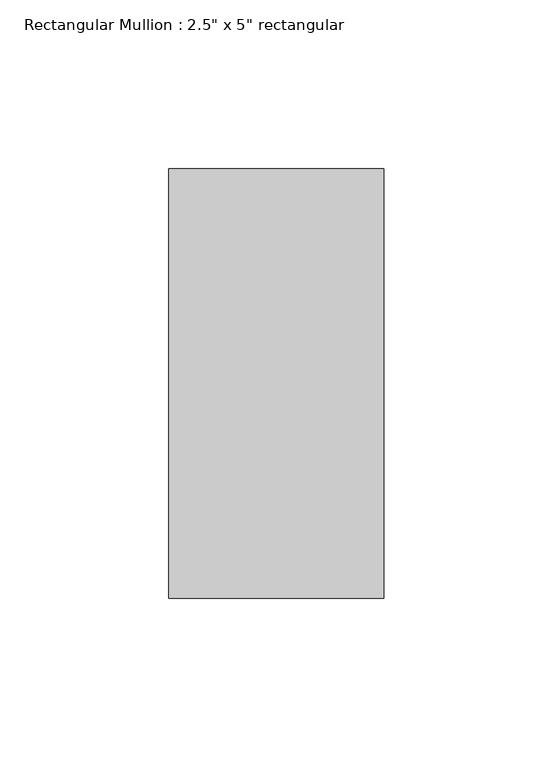
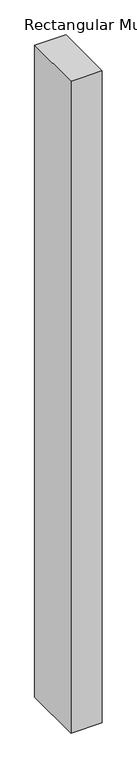
"""IFC4 building model written with IfcOpenShell, lengths in millimetres: member geometry."""

from ifc_helpers import new_model, si_unit, frame, origin, place, context, project, spatial, polyline, outline, extrude, source, transform, mapped, element, save


def member_07d47f19(model_context):
    return source(origin(), model_context, "Body", "SweptSolid", [
        extrude(outline(polyline([(31.75, 63.5), (31.75, -63.5), (-31.75, -63.5), (-31.75, 63.5), (31.75, 63.5)])), frame((0.0, 0.0, -1397.0), z_axis=(0.0, 0.0, 1.0), x_axis=(1.0, 0.0, 0.0)), (0.0, 0.0, 1.0), 1397.0),
    ])


if __name__ == "__main__":
    model = new_model("IFC4")
    model_context = context("Model", 3, world=origin())
    ifc_project = project(units=[si_unit("LENGTHUNIT", "METRE", prefix="MILLI")], contexts=[model_context])
    site = spatial("IfcSite", under=ifc_project)
    building = spatial("IfcBuilding", under=site)
    placement = place(None, origin())
    member_shape = member_07d47f19(model_context)
    element("IfcMember", 1, ObjectType="Rectangular Mullion : 2.5\" x 5\" rectangular", at=placement, inside=building, context=model_context, shape_type="MappedRepresentation", body=[
        mapped(member_shape, transform((0.0, 0.0, 0.0), x_axis=(1.0, 0.0, 0.0), y_axis=(0.0, 1.0, 0.0), z_axis=(0.0, 0.0, 1.0))),
    ])
    save(model, "model.ifc")

# Revit data of these elements
# Type "Rectangular Mullion : 2.5\" x 5\" rectangular"
#   built-in parameter 1007304 = 0.416667 (stored number, unit not read)
#   built-in parameter 1007301 = 0.104167 (stored number, unit not read)
#   built-in parameter 1007300 = 0.104167 (stored number, unit not read)
